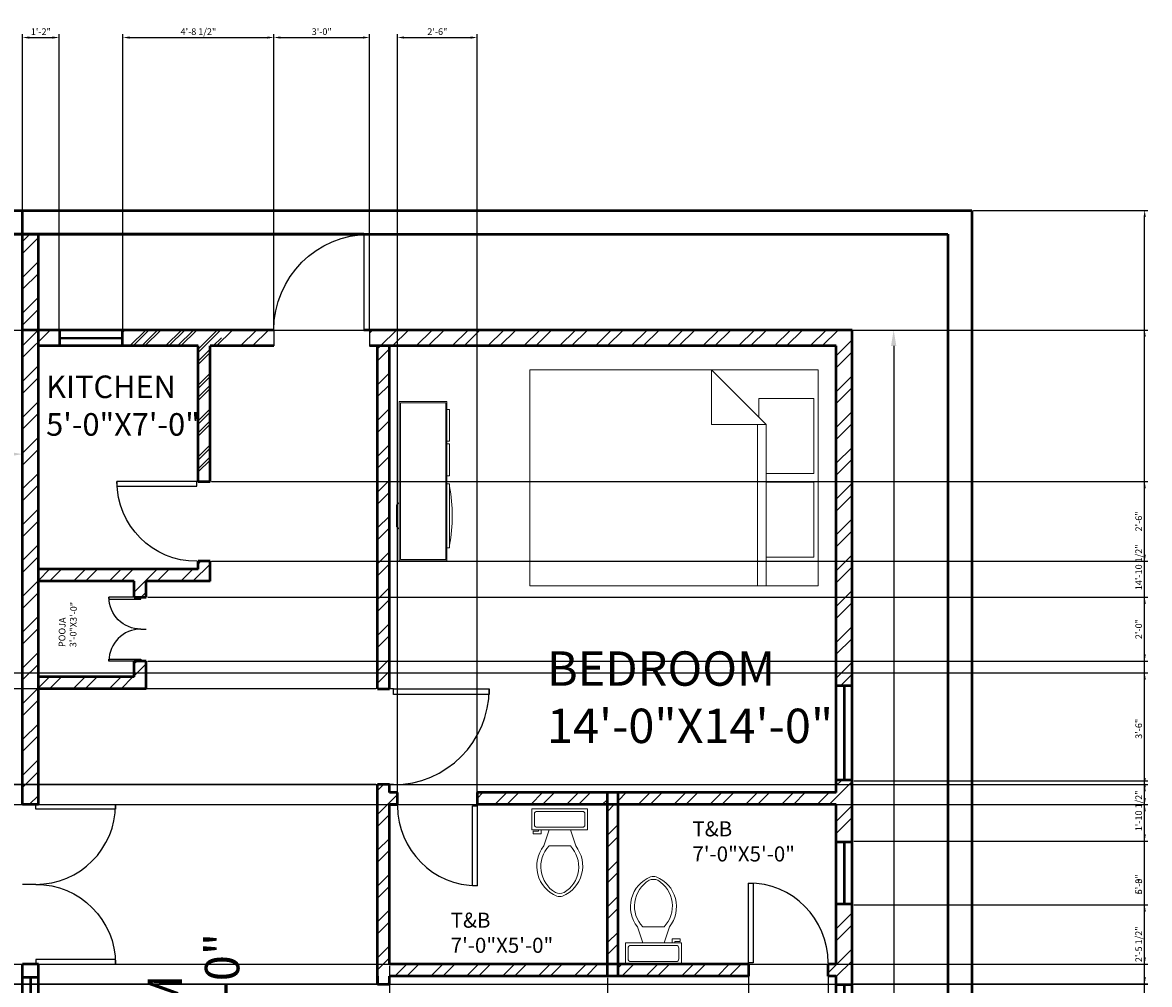
# Model space of a CAD drawing. Units: inches. Extents: x -12550 to 6516, y 1273 to 18700.
# Tile 7 of 19: x 2426 to 2849, y 2227 to 2589. Entities that reach past the tile are written whole.
import ezdxf

# ---------------------------------------------------------------- set-up
doc = ezdxf.new("R2010")
doc.units = ezdxf.units.IN
for name, color, linetype, lineweight in [('A-ANNO-DIMS', 2, 'Continuous', 18), ('A-AREA-IDEN', 1, 'Continuous', 18), ('A-DOOR', 5, 'Continuous', 25), ('A-FURN', 8, 'Continuous', 18), ('A-GLAZ', 3, 'Continuous', 25), ('A-WALL', 7, 'Continuous', 50), ('A-WALL-PATT', 8, 'Continuous', 13)]:
    doc.layers.add(name, color=color, linetype=linetype, lineweight=lineweight)
doc.styles.get("Standard").update_dxf_attribs({"font": 'arial.ttf'})
doc.dimstyles.new('ISO-25', dxfattribs={"dimtxt": 2.5, "dimasz": 2.5, "dimexe": 1.25, "dimexo": 0.625, "dimtad": 1, "dimlunit": 4, "dimtxsty": 'Standard', "dimcen": 2.5, "dimadec": 0, "dimazin": 0, "dimtfac": 1, "dimtmove": 0, "dimatfit": 3, "dimfxl": 1, "dimarcsym": 0})
pattern_1 = [(45, (-2e-13, 567), (-6.735192, 6.735192), []), (45, (4.49, 567), (-6.735192, 6.735192), [])]

# ---------------------------------------------------------------- blocks, each defined once
blk = doc.blocks.new('*U2')
for p, q in [((0, 0), (0, -5)), ((30, 0), (30, -5))]:
    blk.add_line(p, q)
blk.add_lwpolyline([(0, 0), (0, 30), (1.75, 30), (1.75, 0)], close=True)
blk.add_arc((0, 0), 30, 0, 90)
blk = doc.blocks.new('Bed - Queen')
for p, q in [((0, -80.00003), (0, 0)), ((0, 0), (59.99999, 0)), ((59.99999, 0), (59.99999, -80.00003)), ((7.99999, -1.2), (28.79998, -1.2)), ((7.99999, -14.4), (7.99999, -1.2)), ((28.79998, -1.2), (28.79998, -14.4)), ((31.19999, -1.2), (51.99999, -1.2)), ((31.19999, -14.4), (31.19999, -1.2)), ((51.99999, -1.2), (51.99999, -16.4)), ((0, -14.4), (44.8, -14.4)), ((59.99999, -29.6), (44.8, -14.4)), ((44.8, -14.4), (44.8, -29.6)), ((44.8, -16.8), (0, -16.8)), ((51.99999, -16.4), (46.79936, -16.4)), ((44.8, -29.6), (59.99999, -29.6)), ((59.99999, -80.00003), (0, -80.00003))]:
    blk.add_line(p, q)
blk = doc.blocks.new('Toilet - top')
for p, q in [((9.5, -6), (9.5, -2)), ((-8, -8.5), (-8, -8)), ((-7, -8), (-7, -9.5)), ((-4, -8), (-6, -14)), ((4, -8), (6, -14)), ((-10, -8.5), (-8, -8.5)), ((-10, -9.5), (-10, -8.5)), ((-7, -9.5), (-10, -9.5)), ((4, -14), (-4, -14))]:
    blk.add_line(p, q)
blk.add_lwpolyline([(10.5, -8), (10.5, 0), (-10.5, 0), (-10.5, -8)], close=True)
for points in [[(-9.5, -2), (-9.5, -6)], [(8.5, -1), (-8.5, -1)], [(-8.5, -7), (8.5, -7)]]:
    blk.add_lwpolyline(points)
for centre, radius, start, end in [((-8.62, -1.88), 0.884, 81.8699, 188.1301), ((8.62, -1.88), 0.884, 351.8699, 98.1301), ((-8.62, -6.12), 0.884, 171.8699, 278.1301), ((8.62, -6.12), 0.884, 261.8699, 8.1301), ((3.52, -21.58), 12.17, 141.4691, 247.9714), ((4.2, -21.82), 11.33, 136.3677, 238.9468), ((-3.52, -21.58), 12.17, 292.0284, 38.5307), ((-4.2, -21.82), 11.33, 301.053, 43.6321), ((0, -27.88), 4, 245.7318, 294.2682), ((0, -29), 4, 254.8605, 285.1395)]:
    blk.add_arc(centre, radius, start, end)
blk = doc.blocks.new('Entertainment Center')
for p, q in [((-4, 0), (-5, -1)), ((4, 0), (-4, 0)), ((5, -1), (4, 0)), ((-17, -19), (-17, -1)), ((-17, -1), (43, -1)), ((-16.5, -18.5), (-16.5, -1.5)), ((-16.5, -1.5), (42.5, -1.5)), ((42.5, -1.5), (42.5, -18.5)), ((43, -1), (43, -19)), ((43, -19), (-17, -19)), ((42.5, -18.5), (-16.5, -18.5)), ((-12, -20), (-12, -19)), ((12, -20), (-12, -20)), ((12, -19), (12, -20)), ((15, -20), (15, -19)), ((27, -20), (15, -20)), ((27, -19), (27, -20)), ((28, -20), (28, -19)), ((40, -20), (28, -20)), ((40, -19), (40, -20))]:
    blk.add_line(p, q)
blk.add_arc((0, 40), 61, 259.6111, 280.3889)
blk = doc.blocks.new('*D16')
at = {"layer": 'A-ANNO-DIMS', "color": 0, "lineweight": -2, "transparency": 16777216}
for p, q in [((2738.31, 2473.25), (2754.56, 2473.25)), ((2753.31, 2467.25), (2753.31, 1495.25)), ((2738.31, 1489.25), (2754.56, 1489.25))]:
    blk.add_line(p, q, dxfattribs=at)
at = {"layer": 'A-ANNO-DIMS', "color": 0, "transparency": 16777216}
for points in [[(2752.31, 2467.25), (2754.31, 2467.25), (2753.31, 2473.25)], [(2752.31, 1495.25), (2754.31, 1495.25), (2753.31, 1489.25)]]:
    blk.add_solid(points, dxfattribs=at)
at = {"layer": 'Defpoints', "color": 0, "transparency": 16777216}
for p in [(2737.69, 2473.25), (2737.69, 1489.25), (2753.31, 1489.25)]:
    blk.add_point(p, dxfattribs=at)
at = {"layer": 'A-ANNO-DIMS', "color": 0, "transparency": 16777216, "insert": (2749.62, 1981.25), "char_height": 6, "attachment_point": 5, "rotation": 90}
blk.add_mtext("82'", dxfattribs=at)
blk = doc.blocks.new('*D19')
at = {"layer": 'A-ANNO-DIMS', "color": 0, "lineweight": -2, "transparency": 16777216}
for p, q in [((2329.69, 2407.12), (2329.69, 2427.81)), ((2335.69, 2426.56), (2419.69, 2426.56)), ((2425.69, 2407.12), (2425.69, 2427.81))]:
    blk.add_line(p, q, dxfattribs=at)
at = {"layer": 'A-ANNO-DIMS', "color": 0, "transparency": 16777216}
for points in [[(2335.69, 2427.56), (2335.69, 2425.56), (2329.69, 2426.56)], [(2419.69, 2427.56), (2419.69, 2425.56), (2425.69, 2426.56)]]:
    blk.add_solid(points, dxfattribs=at)
at = {"layer": 'Defpoints', "color": 0, "transparency": 16777216}
for p in [(2425.69, 2426.56), (2329.69, 2406.5), (2425.69, 2406.5)]:
    blk.add_point(p, dxfattribs=at)
at = {"layer": 'A-ANNO-DIMS', "color": 0, "transparency": 16777216, "insert": (2377.69, 2430.25), "char_height": 6, "attachment_point": 5}
blk.add_mtext("8'", dxfattribs=at)
blk = doc.blocks.new('WIN-3FT')
for p, q in [((0, 0), (0, 6)), ((0, 6), (36.02, 6)), ((0.5, 0), (0.5, 6)), ((35.52, 6), (35.52, 0)), ((36.02, 6), (36.02, 0)), ((36.02, 0), (0, 0)), ((35.52, 3.2), (0.5, 3.2)), ((35.52, 2.8), (0.5, 2.8))]:
    blk.add_line(p, q)
blk = doc.blocks.new('WIN-2FT')
for p, q in [((0, 0), (0, 24.02)), ((0, 24.02), (6, 24.02)), ((0, 23.52), (6, 23.52)), ((2.8, 0.5), (2.8, 23.52)), ((3.2, 0.5), (3.2, 23.52)), ((6, 24.02), (6, 0)), ((6, 0.5), (0, 0.5)), ((6, 0), (0, 0))]:
    blk.add_line(p, q)
blk = doc.blocks.new('*D95')
at = {"layer": 'A-ANNO-DIMS', "color": 0, "lineweight": -2, "transparency": 16777216}
for p, q in [((2783.31, 2518.25), (2848.94, 2518.25)), ((2847.69, 1446.75), (2847.69, 2515.75)), ((2783.31, 1444.25), (2848.94, 1444.25))]:
    blk.add_line(p, q, dxfattribs=at)
at = {"layer": 'A-ANNO-DIMS', "color": 0, "transparency": 16777216}
for points in [[(2847.27, 2515.75), (2848.11, 2515.75), (2847.69, 2518.25)], [(2847.27, 1446.75), (2848.11, 1446.75), (2847.69, 1444.25)]]:
    blk.add_solid(points, dxfattribs=at)
at = {"layer": 'Defpoints', "color": 0, "transparency": 16777216}
for p in [(2782.69, 2518.25), (2847.69, 2518.25), (2782.69, 1444.25)]:
    blk.add_point(p, dxfattribs=at)
at = {"layer": 'A-ANNO-DIMS', "color": 0, "transparency": 16777216, "insert": (2845.79, 1981.25), "char_height": 2.5, "attachment_point": 5, "rotation": 90}
blk.add_mtext('89\'-6"', dxfattribs=at)
blk = doc.blocks.new('*D139')
at = {"layer": 'A-ANNO-DIMS', "color": 0, "lineweight": -2, "transparency": 16777216}
for p, q in [((2196.81, 2302.25), (2848.94, 2302.25)), ((2847.69, 2229.75), (2847.69, 2299.75)), ((2196.81, 2227.25), (2848.94, 2227.25))]:
    blk.add_line(p, q, dxfattribs=at)
at = {"layer": 'A-ANNO-DIMS', "color": 0, "transparency": 16777216}
for points in [[(2847.27, 2299.75), (2848.11, 2299.75), (2847.69, 2302.25)], [(2847.27, 2229.75), (2848.11, 2229.75), (2847.69, 2227.25)]]:
    blk.add_solid(points, dxfattribs=at)
at = {"layer": 'Defpoints', "color": 0, "transparency": 16777216}
for p in [(2196.19, 2302.25), (2847.69, 2302.25), (2196.19, 2227.25)]:
    blk.add_point(p, dxfattribs=at)
at = {"layer": 'A-ANNO-DIMS', "color": 0, "transparency": 16777216, "insert": (2845.79, 2264.75), "char_height": 2.5, "attachment_point": 5, "rotation": 90}
blk.add_mtext('6\'-3"', dxfattribs=at)
blk = doc.blocks.new('*D140')
at = {"layer": 'A-ANNO-DIMS', "color": 0, "lineweight": -2, "transparency": 16777216}
for p, q in [((2196.81, 2344.25), (2848.94, 2344.25)), ((2847.69, 2304.75), (2847.69, 2341.75)), ((2196.81, 2302.25), (2848.94, 2302.25))]:
    blk.add_line(p, q, dxfattribs=at)
at = {"layer": 'A-ANNO-DIMS', "color": 0, "transparency": 16777216}
for points in [[(2847.27, 2341.75), (2848.11, 2341.75), (2847.69, 2344.25)], [(2847.27, 2304.75), (2848.11, 2304.75), (2847.69, 2302.25)]]:
    blk.add_solid(points, dxfattribs=at)
at = {"layer": 'Defpoints', "color": 0, "transparency": 16777216}
for p in [(2196.19, 2344.25), (2847.69, 2344.25), (2196.19, 2302.25)]:
    blk.add_point(p, dxfattribs=at)
at = {"layer": 'A-ANNO-DIMS', "color": 0, "transparency": 16777216, "insert": (2845.79, 2323.25), "char_height": 2.5, "attachment_point": 5, "rotation": 90}
blk.add_mtext('3\'-6"', dxfattribs=at)
blk = doc.blocks.new('*D144')
at = {"layer": 'A-ANNO-DIMS', "color": 0, "lineweight": -2, "transparency": 16777216}
for p, q in [((2330.31, 2294.75), (2848.94, 2294.75)), ((2847.69, 2237.25), (2847.69, 2292.25)), ((2330.31, 2234.75), (2848.94, 2234.75))]:
    blk.add_line(p, q, dxfattribs=at)
at = {"layer": 'A-ANNO-DIMS', "color": 0, "transparency": 16777216}
for points in [[(2847.27, 2292.25), (2848.11, 2292.25), (2847.69, 2294.75)], [(2847.27, 2237.25), (2848.11, 2237.25), (2847.69, 2234.75)]]:
    blk.add_solid(points, dxfattribs=at)
at = {"layer": 'Defpoints', "color": 0, "transparency": 16777216}
for p in [(2329.69, 2294.75), (2847.69, 2294.75), (2329.69, 2234.75)]:
    blk.add_point(p, dxfattribs=at)
at = {"layer": 'A-ANNO-DIMS', "color": 0, "transparency": 16777216, "insert": (2845.79, 2264.75), "char_height": 2.5, "attachment_point": 5, "rotation": 90}
blk.add_mtext('5\'-0"', dxfattribs=at)
blk = doc.blocks.new('*D146')
at = {"layer": 'A-ANNO-DIMS', "color": 0, "lineweight": -2, "transparency": 16777216}
for p, q in [((2330.31, 2473.25), (2848.94, 2473.25)), ((2847.69, 2297.25), (2847.69, 2470.75)), ((2330.31, 2294.75), (2848.94, 2294.75))]:
    blk.add_line(p, q, dxfattribs=at)
at = {"layer": 'A-ANNO-DIMS', "color": 0, "transparency": 16777216}
for points in [[(2847.27, 2470.75), (2848.11, 2470.75), (2847.69, 2473.25)], [(2847.27, 2297.25), (2848.11, 2297.25), (2847.69, 2294.75)]]:
    blk.add_solid(points, dxfattribs=at)
at = {"layer": 'Defpoints', "color": 0, "transparency": 16777216}
for p in [(2329.69, 2473.25), (2847.69, 2473.25), (2329.69, 2294.75)]:
    blk.add_point(p, dxfattribs=at)
at = {"layer": 'A-ANNO-DIMS', "color": 0, "transparency": 16777216, "insert": (2845.77, 2384), "char_height": 2.5, "attachment_point": 5, "rotation": 90}
blk.add_mtext('14\'-10 1/2"', dxfattribs=at)
blk = doc.blocks.new('*D149')
at = {"layer": 'A-ANNO-DIMS', "color": 0, "lineweight": -2, "transparency": 16777216}
for p, q in [((2425.69, 2473.87), (2425.69, 2584.5)), ((2428.19, 2583.25), (2436.95, 2583.25)), ((2439.45, 2473.87), (2439.45, 2584.5))]:
    blk.add_line(p, q, dxfattribs=at)
at = {"layer": 'A-ANNO-DIMS', "color": 0, "transparency": 16777216}
for points in [[(2428.19, 2583.66), (2428.19, 2582.83), (2425.69, 2583.25)], [(2436.95, 2583.66), (2436.95, 2582.83), (2439.45, 2583.25)]]:
    blk.add_solid(points, dxfattribs=at)
at = {"layer": 'Defpoints', "color": 0, "transparency": 16777216}
for p in [(2439.45, 2583.25), (2425.69, 2473.25), (2439.45, 2473.25)]:
    blk.add_point(p, dxfattribs=at)
at = {"layer": 'A-ANNO-DIMS', "color": 0, "transparency": 16777216, "insert": (2432.57, 2585.13), "char_height": 2.5, "attachment_point": 5}
blk.add_mtext('1\'-2"', dxfattribs=at)
blk = doc.blocks.new('*D150')
at = {"layer": 'A-ANNO-DIMS', "color": 0, "lineweight": -2, "transparency": 16777216}
for p, q in [((2463.46, 2473.87), (2463.46, 2584.5)), ((2465.96, 2583.25), (2517.69, 2583.25)), ((2520.19, 2473.87), (2520.19, 2584.5))]:
    blk.add_line(p, q, dxfattribs=at)
at = {"layer": 'A-ANNO-DIMS', "color": 0, "transparency": 16777216}
for points in [[(2465.96, 2583.66), (2465.96, 2582.83), (2463.46, 2583.25)], [(2517.69, 2583.66), (2517.69, 2582.83), (2520.19, 2583.25)]]:
    blk.add_solid(points, dxfattribs=at)
at = {"layer": 'Defpoints', "color": 0, "transparency": 16777216}
for p in [(2520.19, 2583.25), (2463.46, 2473.25), (2520.19, 2473.25)]:
    blk.add_point(p, dxfattribs=at)
at = {"layer": 'A-ANNO-DIMS', "color": 0, "transparency": 16777216, "insert": (2491.83, 2585.16), "char_height": 2.5, "attachment_point": 5}
blk.add_mtext('4\'-8 1/2"', dxfattribs=at)
blk = doc.blocks.new('*D151')
at = {"layer": 'A-ANNO-DIMS', "color": 0, "lineweight": -2, "transparency": 16777216}
for p, q in [((2520.19, 2473.87), (2520.19, 2584.5)), ((2522.69, 2583.25), (2553.69, 2583.25)), ((2556.19, 2473.87), (2556.19, 2584.5))]:
    blk.add_line(p, q, dxfattribs=at)
at = {"layer": 'A-ANNO-DIMS', "color": 0, "transparency": 16777216}
for points in [[(2522.69, 2583.66), (2522.69, 2582.83), (2520.19, 2583.25)], [(2553.69, 2583.66), (2553.69, 2582.83), (2556.19, 2583.25)]]:
    blk.add_solid(points, dxfattribs=at)
at = {"layer": 'Defpoints', "color": 0, "transparency": 16777216}
for p in [(2556.19, 2583.25), (2520.19, 2473.25), (2556.19, 2473.25)]:
    blk.add_point(p, dxfattribs=at)
at = {"layer": 'A-ANNO-DIMS', "color": 0, "transparency": 16777216, "insert": (2538.19, 2585.15), "char_height": 2.5, "attachment_point": 5}
blk.add_mtext('3\'-0"', dxfattribs=at)
blk = doc.blocks.new('*D155')
at = {"layer": 'A-ANNO-DIMS', "color": 0, "lineweight": -2, "transparency": 16777216}
for p, q in [((2738.31, 2257.02), (2848.94, 2257.02)), ((2847.69, 2229.87), (2847.69, 2254.52)), ((2738.31, 2227.37), (2848.94, 2227.37))]:
    blk.add_line(p, q, dxfattribs=at)
at = {"layer": 'A-ANNO-DIMS', "color": 0, "transparency": 16777216}
for points in [[(2847.27, 2254.52), (2848.11, 2254.52), (2847.69, 2257.02)], [(2847.27, 2229.87), (2848.11, 2229.87), (2847.69, 2227.37)]]:
    blk.add_solid(points, dxfattribs=at)
at = {"layer": 'Defpoints', "color": 0, "transparency": 16777216}
for p in [(2737.69, 2257.02), (2847.69, 2257.02), (2737.69, 2227.37)]:
    blk.add_point(p, dxfattribs=at)
at = {"layer": 'A-ANNO-DIMS', "color": 0, "transparency": 16777216, "insert": (2845.77, 2242.2), "char_height": 2.5, "attachment_point": 5, "rotation": 90}
blk.add_mtext('2\'-5 1/2"', dxfattribs=at)
blk = doc.blocks.new('*D156')
at = {"layer": 'A-ANNO-DIMS', "color": 0, "lineweight": -2, "transparency": 16777216}
for p, q in [((2738.31, 2303.73), (2848.94, 2303.73)), ((2847.69, 2283.54), (2847.69, 2301.23)), ((2738.31, 2281.04), (2848.94, 2281.04))]:
    blk.add_line(p, q, dxfattribs=at)
at = {"layer": 'A-ANNO-DIMS', "color": 0, "transparency": 16777216}
for points in [[(2847.27, 2301.23), (2848.11, 2301.23), (2847.69, 2303.73)], [(2847.27, 2283.54), (2848.11, 2283.54), (2847.69, 2281.04)]]:
    blk.add_solid(points, dxfattribs=at)
at = {"layer": 'Defpoints', "color": 0, "transparency": 16777216}
for p in [(2737.69, 2303.73), (2847.69, 2303.73), (2737.69, 2281.04)]:
    blk.add_point(p, dxfattribs=at)
at = {"layer": 'A-ANNO-DIMS', "color": 0, "transparency": 16777216, "insert": (2845.77, 2292.39), "char_height": 2.5, "attachment_point": 5, "rotation": 90}
blk.add_mtext('1\'-10 1/2"', dxfattribs=at)
blk = doc.blocks.new('*D158')
at = {"layer": 'A-ANNO-DIMS', "color": 0, "lineweight": -2, "transparency": 16777216}
for p, q in [((2558.56, 2227.25), (1906.44, 2227.25)), ((1907.69, 2193.75), (1907.69, 2224.75)), ((2558.56, 2191.25), (1906.44, 2191.25))]:
    blk.add_line(p, q, dxfattribs=at)
at = {"layer": 'A-ANNO-DIMS', "color": 0, "transparency": 16777216}
for points in [[(1907.27, 2224.75), (1908.11, 2224.75), (1907.69, 2227.25)], [(1907.27, 2193.75), (1908.11, 2193.75), (1907.69, 2191.25)]]:
    blk.add_solid(points, dxfattribs=at)
at = {"layer": 'Defpoints', "color": 0, "transparency": 16777216}
for p in [(1907.69, 2227.25), (2559.19, 2227.25), (2559.19, 2191.25)]:
    blk.add_point(p, dxfattribs=at)
at = {"layer": 'A-ANNO-DIMS', "color": 0, "transparency": 16777216, "insert": (1905.79, 2209.25), "char_height": 2.5, "attachment_point": 5, "rotation": 90}
blk.add_mtext('3\'-0"', dxfattribs=at)
blk = doc.blocks.new('*D159')
at = {"layer": 'A-ANNO-DIMS', "color": 0, "lineweight": -2, "transparency": 16777216}
for p, q in [((2558.56, 2302.25), (1906.44, 2302.25)), ((1907.69, 2229.75), (1907.69, 2299.75)), ((2558.56, 2227.25), (1906.44, 2227.25))]:
    blk.add_line(p, q, dxfattribs=at)
at = {"layer": 'A-ANNO-DIMS', "color": 0, "transparency": 16777216}
for points in [[(1907.27, 2299.75), (1908.11, 2299.75), (1907.69, 2302.25)], [(1907.27, 2229.75), (1908.11, 2229.75), (1907.69, 2227.25)]]:
    blk.add_solid(points, dxfattribs=at)
at = {"layer": 'Defpoints', "color": 0, "transparency": 16777216}
for p in [(1907.69, 2302.25), (2559.19, 2302.25), (2559.19, 2227.25)]:
    blk.add_point(p, dxfattribs=at)
at = {"layer": 'A-ANNO-DIMS', "color": 0, "transparency": 16777216, "insert": (1905.79, 2264.75), "char_height": 2.5, "attachment_point": 5, "rotation": 90}
blk.add_mtext('6\'-3"', dxfattribs=at)
blk = doc.blocks.new('*D160')
at = {"layer": 'A-ANNO-DIMS', "color": 0, "lineweight": -2, "transparency": 16777216}
for p, q in [((2558.56, 2338.25), (1906.44, 2338.25)), ((1907.69, 2304.75), (1907.69, 2335.75)), ((2558.56, 2302.25), (1906.44, 2302.25))]:
    blk.add_line(p, q, dxfattribs=at)
at = {"layer": 'A-ANNO-DIMS', "color": 0, "transparency": 16777216}
for points in [[(1907.27, 2335.75), (1908.11, 2335.75), (1907.69, 2338.25)], [(1907.27, 2304.75), (1908.11, 2304.75), (1907.69, 2302.25)]]:
    blk.add_solid(points, dxfattribs=at)
at = {"layer": 'Defpoints', "color": 0, "transparency": 16777216}
for p in [(1907.69, 2338.25), (2559.19, 2338.25), (2559.19, 2302.25)]:
    blk.add_point(p, dxfattribs=at)
at = {"layer": 'A-ANNO-DIMS', "color": 0, "transparency": 16777216, "insert": (1905.79, 2320.25), "char_height": 2.5, "attachment_point": 5, "rotation": 90}
blk.add_mtext('3\'-0"', dxfattribs=at)
blk = doc.blocks.new('*D161')
at = {"layer": 'A-ANNO-DIMS', "color": 0, "lineweight": -2, "transparency": 16777216}
for p, q in [((2566.69, 2295.37), (2566.69, 2584.5)), ((2569.19, 2583.25), (2594.19, 2583.25)), ((2596.69, 2295.37), (2596.69, 2584.5))]:
    blk.add_line(p, q, dxfattribs=at)
at = {"layer": 'A-ANNO-DIMS', "color": 0, "transparency": 16777216}
for points in [[(2569.19, 2583.66), (2569.19, 2582.83), (2566.69, 2583.25)], [(2594.19, 2583.66), (2594.19, 2582.83), (2596.69, 2583.25)]]:
    blk.add_solid(points, dxfattribs=at)
at = {"layer": 'Defpoints', "color": 0, "transparency": 16777216}
for p in [(2596.69, 2583.25), (2566.69, 2294.75), (2596.69, 2294.75)]:
    blk.add_point(p, dxfattribs=at)
at = {"layer": 'A-ANNO-DIMS', "color": 0, "transparency": 16777216, "insert": (2581.69, 2585.15), "char_height": 2.5, "attachment_point": 5}
blk.add_mtext('2\'-6"', dxfattribs=at)
blk = doc.blocks.new('*D162')
at = {"layer": 'A-ANNO-DIMS', "color": 0, "lineweight": -2, "transparency": 16777216}
for p, q in [((2698.69, 2234.12), (2698.69, 1378)), ((2728.69, 2234.12), (2728.69, 1378)), ((2701.19, 1379.25), (2726.19, 1379.25))]:
    blk.add_line(p, q, dxfattribs=at)
at = {"layer": 'A-ANNO-DIMS', "color": 0, "transparency": 16777216}
for points in [[(2701.19, 1379.66), (2701.19, 1378.83), (2698.69, 1379.25)], [(2726.19, 1379.66), (2726.19, 1378.83), (2728.69, 1379.25)]]:
    blk.add_solid(points, dxfattribs=at)
at = {"layer": 'Defpoints', "color": 0, "transparency": 16777216}
for p in [(2698.69, 2234.75), (2728.69, 2234.75), (2728.69, 1379.25)]:
    blk.add_point(p, dxfattribs=at)
at = {"layer": 'A-ANNO-DIMS', "color": 0, "transparency": 16777216, "insert": (2713.69, 1381.15), "char_height": 2.5, "attachment_point": 5}
blk.add_mtext('2\'-6"', dxfattribs=at)
blk = doc.blocks.new('*D163')
at = {"layer": 'A-ANNO-DIMS', "color": 0, "lineweight": -2, "transparency": 16777216}
for p, q in [((2563.69, 2234.12), (2563.69, 1378)), ((2645.69, 2229.62), (2645.69, 1378)), ((2566.19, 1379.25), (2643.19, 1379.25))]:
    blk.add_line(p, q, dxfattribs=at)
at = {"layer": 'A-ANNO-DIMS', "color": 0, "transparency": 16777216}
for points in [[(2566.19, 1379.66), (2566.19, 1378.83), (2563.69, 1379.25)], [(2643.19, 1379.66), (2643.19, 1378.83), (2645.69, 1379.25)]]:
    blk.add_solid(points, dxfattribs=at)
at = {"layer": 'Defpoints', "color": 0, "transparency": 16777216}
for p in [(2563.69, 2234.75), (2645.69, 2230.25), (2645.69, 1379.25)]:
    blk.add_point(p, dxfattribs=at)
at = {"layer": 'A-ANNO-DIMS', "color": 0, "transparency": 16777216, "insert": (2604.69, 1381.15), "char_height": 2.5, "attachment_point": 5}
blk.add_mtext('6\'-10"', dxfattribs=at)
blk = doc.blocks.new('*D167')
at = {"layer": 'A-ANNO-DIMS', "color": 0, "lineweight": -2, "transparency": 16777216}
for p, q in [((2496.81, 2416.25), (2848.94, 2416.25)), ((2847.69, 2388.75), (2847.69, 2413.75)), ((2496.81, 2386.25), (2848.94, 2386.25))]:
    blk.add_line(p, q, dxfattribs=at)
at = {"layer": 'A-ANNO-DIMS', "color": 0, "transparency": 16777216}
for points in [[(2847.27, 2413.75), (2848.11, 2413.75), (2847.69, 2416.25)], [(2847.27, 2388.75), (2848.11, 2388.75), (2847.69, 2386.25)]]:
    blk.add_solid(points, dxfattribs=at)
at = {"layer": 'Defpoints', "color": 0, "transparency": 16777216}
for p in [(2496.19, 2416.25), (2847.69, 2416.25), (2496.19, 2386.25)]:
    blk.add_point(p, dxfattribs=at)
at = {"layer": 'A-ANNO-DIMS', "color": 0, "transparency": 16777216, "insert": (2845.79, 2401.25), "char_height": 2.5, "attachment_point": 5, "rotation": 90}
blk.add_mtext('2\'-6"', dxfattribs=at)
blk = doc.blocks.new('*D168')
at = {"layer": 'A-ANNO-DIMS', "color": 0, "lineweight": -2, "transparency": 16777216}
for p, q in [((2472.81, 2372.75), (2848.94, 2372.75)), ((2847.69, 2351.25), (2847.69, 2370.25)), ((2472.81, 2348.75), (2848.94, 2348.75))]:
    blk.add_line(p, q, dxfattribs=at)
at = {"layer": 'A-ANNO-DIMS', "color": 0, "transparency": 16777216}
for points in [[(2847.27, 2370.25), (2848.11, 2370.25), (2847.69, 2372.75)], [(2847.27, 2351.25), (2848.11, 2351.25), (2847.69, 2348.75)]]:
    blk.add_solid(points, dxfattribs=at)
at = {"layer": 'Defpoints', "color": 0, "transparency": 16777216}
for p in [(2472.19, 2372.75), (2847.69, 2372.75), (2472.19, 2348.75)]:
    blk.add_point(p, dxfattribs=at)
at = {"layer": 'A-ANNO-DIMS', "color": 0, "transparency": 16777216, "insert": (2845.79, 2360.75), "char_height": 2.5, "attachment_point": 5, "rotation": 90}
blk.add_mtext('2\'-0"', dxfattribs=at)

msp = doc.modelspace()

# ---------------------------------------------------------------- hatches: boundary and pattern name
at = {"layer": 'A-WALL-PATT'}
h = msp.add_hatch(dxfattribs=at)
h.set_pattern_fill('ANSI32', color=256)
h.paths.add_polyline_path([(2431.689, 2509.247), (2425.689, 2509.247), (2425.689, 2473.247), (2431.689, 2473.247)])
h = msp.add_hatch(dxfattribs=at)
h.set_pattern_fill('ANSI32', color=256)
h.set_pattern_definition(pattern_1)
h.paths.add_polyline_path([(2439.446, 2473.247), (2425.689, 2473.247), (2425.689, 2294.747), (2430.689, 2294.747), (2431.689, 2294.747), (2431.689, 2467.247), (2439.446, 2467.247)])
h = msp.add_hatch(dxfattribs=at)
h.set_pattern_fill('ANSI32', color=256)
h.set_pattern_definition(pattern_1)
h.paths.add_polyline_path([(2500.528, 2473.247), (2463.463, 2473.247), (2463.463, 2467.247), (2491.689, 2467.247), (2491.689, 2416.247), (2496.189, 2416.247), (2496.189, 2467.247), (2500.528, 2467.247)])
h = msp.add_hatch(dxfattribs=at)
h.set_pattern_fill('ANSI32', color=256)
h.paths.add_polyline_path([(2463.463, 2473.247), (2463.463, 2467.247), (2491.689, 2467.247), (2491.689, 2416.247), (2496.189, 2416.247), (2496.189, 2467.247), (2520.189, 2467.247), (2520.189, 2473.247)])
h = msp.add_hatch(dxfattribs=at)
h.set_pattern_fill('ANSI32', color=256)
h.set_pattern_definition(pattern_1)
h.paths.add_polyline_path([(2556.189, 2473.247), (2556.189, 2467.247), (2731.689, 2467.247), (2731.689, 2339.747), (2737.689, 2339.747), (2737.689, 2473.247)])
h = msp.add_hatch(dxfattribs=at)
h.set_pattern_fill('ANSI32', color=256)
h.set_pattern_definition(pattern_1)
h.paths.add_polyline_path([(2563.689, 2467.247), (2559.189, 2467.247), (2559.189, 2338.247), (2563.689, 2338.247)])
h = msp.add_hatch(dxfattribs=at)
h.set_pattern_fill('ANSI32', color=256)
h.set_pattern_definition(pattern_1)
h.paths.add_polyline_path([(2496.189, 2386.247), (2491.689, 2386.247), (2491.689, 2383.247), (2431.689, 2383.247), (2431.689, 2378.747), (2467.689, 2378.747), (2467.689, 2372.747), (2470.189, 2372.747), (2472.189, 2372.747), (2472.189, 2378.747), (2496.189, 2378.747)])
h = msp.add_hatch(dxfattribs=at)
h.set_pattern_fill('ANSI32', color=256)
h.set_pattern_definition(pattern_1)
h.paths.add_polyline_path([(2472.189, 2348.747), (2470.189, 2348.747), (2467.689, 2348.747), (2467.689, 2342.747), (2431.689, 2342.747), (2431.689, 2338.247), (2472.189, 2338.247)])
h = msp.add_hatch(dxfattribs=at)
h.set_pattern_fill('ANSI32', color=256)
h.set_pattern_definition(pattern_1)
h.paths.add_polyline_path([(2563.689, 2294.747), (2566.689, 2294.747), (2566.689, 2299.247), (2563.689, 2299.247), (2563.689, 2302.247), (2559.189, 2302.247), (2559.189, 2227.247), (2563.689, 2227.247), (2563.689, 2230.247), (2566.641, 2230.247), (2645.689, 2230.247), (2645.689, 2234.747), (2566.641, 2234.747), (2563.689, 2234.747)])
h = msp.add_hatch(dxfattribs=at)
h.set_pattern_fill('ANSI32', color=256)
h.set_pattern_definition(pattern_1)
h.paths.add_polyline_path([(2737.689, 2303.73), (2731.689, 2303.73), (2731.689, 2299.247), (2728.689, 2299.247), (2649.689, 2299.247), (2649.689, 2294.747), (2728.689, 2294.747), (2731.689, 2294.747), (2731.689, 2281.042), (2737.689, 2281.042)])
h = msp.add_hatch(dxfattribs=at)
h.set_pattern_fill('ANSI32', color=256)
h.set_pattern_definition(pattern_1)
h.paths.add_polyline_path([(2645.689, 2299.247), (2596.689, 2299.247), (2596.689, 2294.747), (2645.689, 2294.747)], flags=17)
h = msp.add_hatch(dxfattribs=at)
h.set_pattern_fill('ANSI32', color=256)
h.set_pattern_definition(pattern_1)
h.paths.add_polyline_path([(2649.689, 2294.747), (2645.689, 2294.747), (2645.689, 2234.747), (2649.689, 2234.747)])
h = msp.add_hatch(dxfattribs=at)
h.set_pattern_fill('ANSI32', color=256)
h.set_pattern_definition(pattern_1)
h.paths.add_polyline_path([(2737.689, 2257.024), (2731.689, 2257.024), (2731.689, 2234.747), (2728.689, 2234.747), (2728.689, 2230.247), (2731.689, 2230.247), (2731.689, 2227.369), (2737.689, 2227.369)])
h = msp.add_hatch(dxfattribs=at)
h.set_pattern_fill('ANSI32', color=256)
h.set_pattern_definition(pattern_1)
h.paths.add_polyline_path([(2698.689, 2234.747), (2649.689, 2234.747), (2649.689, 2230.247), (2698.689, 2230.247)])

# ---------------------------------------------------------------- linework, layer by layer
at = {"layer": 'A-WALL'}
for p, q in [((1972.689, 2518.247), (2782.689, 2518.247)), ((2425.689, 2294.747), (2425.689, 2518.247)), ((2782.689, 2518.247), (2782.689, 1444.247)), ((1981.689, 2509.247), (2773.689, 2509.247)), ((2554.089, 2509.247), (2254.089, 2509.247)), ((2431.689, 2294.747), (2431.689, 2509.247)), ((2773.689, 2509.247), (2773.689, 1453.247)), ((2520.189, 2473.247), (2425.689, 2473.247)), ((2559.189, 2473.247), (2554.089, 2473.247)), ((2737.689, 2473.247), (2559.189, 2473.247)), ((2737.689, 2060.923), (2737.689, 2473.247)), ((2491.689, 2467.247), (2431.689, 2467.247)), ((2491.689, 2416.247), (2491.689, 2467.247)), ((2496.189, 2416.247), (2496.189, 2467.247)), ((2520.189, 2467.247), (2496.189, 2467.247)), ((2559.189, 2467.247), (2556.189, 2467.247)), ((2731.689, 2467.247), (2559.189, 2467.247)), ((2559.189, 2338.247), (2559.189, 2467.247)), ((2563.689, 2338.247), (2563.689, 2467.247)), ((2731.689, 2299.247), (2731.689, 2467.247)), ((2491.689, 2416.247), (2496.189, 2416.247)), ((2491.689, 2383.247), (2491.689, 2386.247)), ((2496.189, 2386.247), (2491.689, 2386.247)), ((2496.189, 2378.747), (2496.189, 2386.247)), ((2496.189, 2383.247), (2496.189, 2386.247)), ((2491.689, 2383.247), (2431.689, 2383.247)), ((2467.689, 2378.747), (2431.689, 2378.747)), ((2467.689, 2372.747), (2467.689, 2378.747)), ((2496.189, 2378.747), (2472.189, 2378.747)), ((2472.189, 2372.747), (2472.189, 2378.747)), ((2467.689, 2372.747), (2472.189, 2372.747)), ((2467.689, 2342.747), (2467.689, 2348.747)), ((2472.189, 2348.747), (2467.689, 2348.747)), ((2472.189, 2338.247), (2472.189, 2348.747)), ((2472.189, 2342.747), (2472.189, 2348.747)), ((2467.689, 2342.747), (2431.689, 2342.747)), ((2472.189, 2338.247), (2431.689, 2338.247)), ((2559.189, 2338.247), (2563.689, 2338.247)), ((2559.189, 2227.247), (2559.189, 2302.247)), ((2563.689, 2302.247), (2559.189, 2302.247)), ((2563.689, 2299.247), (2563.689, 2302.247)), ((2563.689, 2299.247), (2563.689, 2302.247)), ((2563.689, 2299.247), (2563.689, 2302.247)), ((2563.689, 2299.247), (2563.689, 2302.247)), ((2566.689, 2299.247), (2563.689, 2299.247)), ((2566.689, 2294.747), (2566.689, 2299.247)), ((2728.689, 2299.247), (2596.689, 2299.247)), ((2596.689, 2299.247), (2596.689, 2294.747)), ((2645.689, 2230.247), (2645.689, 2299.247)), ((2649.689, 2230.247), (2649.689, 2299.247)), ((2731.689, 2299.247), (2728.689, 2299.247)), ((2731.689, 2299.247), (2728.689, 2299.247)), ((2431.689, 2294.747), (2425.689, 2294.747)), ((2566.689, 2294.747), (2563.689, 2294.747)), ((2563.689, 2234.747), (2563.689, 2294.747)), ((2563.689, 2234.747), (2563.689, 2294.747)), ((2563.689, 2234.747), (2563.689, 2294.747)), ((2563.689, 2294.747), (2566.689, 2294.747)), ((2728.689, 2294.747), (2596.689, 2294.747)), ((2731.689, 2294.747), (2728.689, 2294.747)), ((2731.689, 2234.747), (2731.689, 2294.747)), ((2431.689, 2234.747), (2425.689, 2234.747)), ((2425.689, 2056.247), (2425.689, 2234.747)), ((2431.689, 2062.247), (2431.689, 2234.747)), ((2566.641, 2234.747), (2563.689, 2234.747)), ((2698.689, 2234.747), (2566.641, 2234.747)), ((2698.689, 2234.747), (2698.689, 2230.247)), ((2731.689, 2234.747), (2728.689, 2234.747)), ((2728.689, 2230.247), (2728.689, 2234.747)), ((2559.189, 2230.247), (2559.189, 2227.247)), ((2566.641, 2230.247), (2563.689, 2230.247)), ((2563.689, 2227.247), (2563.689, 2230.247)), ((2563.689, 2227.247), (2563.689, 2230.247)), ((2563.689, 2227.247), (2563.689, 2230.247)), ((2698.689, 2230.247), (2566.641, 2230.247)), ((2731.689, 2230.247), (2728.689, 2230.247)), ((2731.689, 2230.247), (2728.689, 2230.247)), ((2731.689, 2062.247), (2731.689, 2230.247)), ((2559.189, 2227.247), (2563.689, 2227.247))]:
    msp.add_line(p, q, dxfattribs=at)

# ---------------------------------------------------------------- block references
at = {"layer": 'A-DOOR', "xscale": -1.199999999999999, "yscale": 1.199999999999999, "zscale": 1.199999999999999}
msp.add_blockref('*U2', (2556.189, 2473.247), dxfattribs=at)
at = {"layer": 'A-DOOR', "xscale": -1}
for p, rotation in [((2491.189, 2416.247), 90), ((2430.689, 2234.747), 270)]:
    msp.add_blockref('*U2', p, dxfattribs=dict(at, rotation=rotation))
at = {"layer": 'A-DOOR'}
for p, xscale, yscale, zscale, rotation in [((2470.189, 2372.747), -0.399999999999997, 0.399999999999997, 0.399999999999997, 90), ((2470.189, 2348.747), 0.399999999999997, 0.399999999999997, 0.399999999999997, 90.00000000000003), ((2565.189, 2338.247), 1.199999999999999, 1.199999999999999, 1.199999999999999, 270)]:
    msp.add_blockref('*U2', p, dxfattribs=dict(at, xscale=xscale, yscale=yscale, zscale=zscale, rotation=rotation))
for p, rotation in [((2596.689, 2294.247), 180), ((2430.689, 2294.747), 270)]:
    msp.add_blockref('*U2', p, dxfattribs=dict(at, rotation=rotation))
msp.add_blockref('*U2', (2698.689, 2235.247), dxfattribs=at)
at = {"layer": 'A-FURN', "xscale": -1.354827908062564, "yscale": 1.354827908062564, "zscale": 1.354827908062564, "rotation": 270}
msp.add_blockref('Bed - Queen', (2724.868, 2376.994), dxfattribs=at)
at = {"layer": 'A-FURN'}
for name, p, rotation in [('Entertainment Center', (2566.318, 2403.379), 89.99999999999999), ('Toilet - top', (2662.958, 2234.747), 180)]:
    msp.add_blockref(name, p, dxfattribs=dict(at, rotation=rotation))
msp.add_blockref('Toilet - top', (2627.711, 2293.198), dxfattribs=at)
at = {"layer": 'A-GLAZ'}
for name, p, rotation in [('WIN-2FT', (2439.446, 2473.247), 269.9999999999959), ('WIN-3FT', (2737.689, 2303.73), 90.00000000000072), ('WIN-2FT', (2737.689, 2281.042), 180), ('WIN-3FT', (2431.689, 2194.032), 90.00000000000047), ('WIN-3FT', (2737.689, 2191.352), 90.00000000000047)]:
    msp.add_blockref(name, p, dxfattribs=dict(at, rotation=rotation))

# ---------------------------------------------------------------- texts
at = {"layer": 'A-AREA-IDEN', "attachment_point": 1}
for s, width, gutter_width, insert, char_height in [('KITCHEN\\P5\'-0"X7\'-0"', 1.29487, 42.422, (2434.569, 2456.124), 8.48435), ('T&B\\P7\'-0"X5\'-0"', 4.19569, 28.328, (2677.611, 2288.465), 5.66556), ('T&B\\P7\'-0"X5\'-0"', 4.19569, 28.328, (2586.701, 2254.107), 5.66556)]:
    msp.add_mtext_dynamic_manual_height_columns(s, width=width, gutter_width=gutter_width, heights=[0], dxfattribs=dict(at, insert=insert, char_height=char_height))
at = {"layer": 'A-AREA-IDEN', "insert": (2439.241, 2354.026), "char_height": 2.5, "attachment_point": 1, "rotation": 89.18385}
msp.add_mtext_dynamic_manual_height_columns('POOJA\\P3\'-0"X3\'-0"', width=0.78585, gutter_width=12.5, heights=[0], dxfattribs=at)
at = {"layer": 'A-AREA-IDEN', "insert": (2622.904, 2352.378), "char_height": 12.93169, "attachment_point": 1}
msp.add_mtext('BEDROOM\\P14\'-0"X14\'-0"', dxfattribs=at)
at = {"layer": 'A-AREA-IDEN', "insert": (2472.713, 2124.153), "char_height": 12.93169, "attachment_point": 1, "rotation": 90}
msp.add_mtext('LIVINGROOM\\P10\'-7.5"X23\'-0"', dxfattribs=at)

# ---------------------------------------------------------------- dimensions: what is measured, and where the dimension line sits
at = {"layer": 'A-ANNO-DIMS'}
for base, p1, p2, override, picture, middle in [((2439.446, 2583.247), (2425.689, 2473.247), (2439.446, 2473.247), {"dimdec": 1, "dimlfac": 1, "dimrnd": 0, "dimzin": 1, "dimdsep": 46, "dimlunit": 4, "dimfrac": 2}, '*D149', (2432.567, 2585.127)), ((2520.189, 2583.247), (2463.463, 2473.247), (2520.189, 2473.247), {"dimdec": 1, "dimlfac": 1, "dimrnd": 0, "dimzin": 1, "dimdsep": 46, "dimlunit": 4, "dimfrac": 2}, '*D150', (2491.826, 2585.165)), ((2556.189, 2583.247), (2520.189, 2473.247), (2556.189, 2473.247), {"dimdec": 1, "dimlfac": 1, "dimrnd": 0, "dimzin": 1, "dimdsep": 46, "dimlunit": 4, "dimfrac": 2}, '*D151', (2538.189, 2585.15)), ((2596.689, 2583.247), (2566.689, 2294.747), (2596.689, 2294.747), {"dimdec": 1, "dimlfac": 1, "dimrnd": 0, "dimzin": 1, "dimdsep": 46, "dimlunit": 4, "dimfrac": 2}, '*D161', (2581.689, 2585.149)), ((2425.689, 2426.562), (2329.689, 2406.497), (2425.689, 2406.497), {"dimtxt": 6, "dimasz": 6, "dimclrd": 0, "dimclre": 0, "dimclrt": 0}, '*D19', (2377.689, 2430.25)), ((2645.689, 1379.247), (2563.689, 2234.747), (2645.689, 2230.247), {"dimdec": 1, "dimlfac": 1, "dimrnd": 0, "dimzin": 1, "dimdsep": 46, "dimlunit": 4, "dimfrac": 2}, '*D163', (2604.689, 1381.149)), ((2728.689, 1379.247), (2698.689, 2234.747), (2728.689, 2234.747), {"dimdec": 1, "dimlfac": 1, "dimrnd": 0, "dimzin": 1, "dimdsep": 46, "dimlunit": 4, "dimfrac": 2}, '*D162', (2713.689, 1381.149))]:
    dim = msp.add_linear_dim(base=base, p1=p1, p2=p2, dimstyle='ISO-25', override=override, dxfattribs=at)
    dim.commit()
    dim.dimension.update_dxf_attribs({"geometry": picture, "text_midpoint": middle})
for base, p1, p2, override, picture, middle in [((2847.689, 2518.247), (2782.689, 1444.247), (2782.689, 2518.247), {"dimdec": 1, "dimlfac": 1, "dimrnd": 0, "dimzin": 1, "dimdsep": 46, "dimlunit": 4, "dimfrac": 2}, '*D95', (2845.787, 1981.247)), ((2847.689, 2473.247), (2329.689, 2294.747), (2329.689, 2473.247), {"dimdec": 1, "dimlfac": 1, "dimrnd": 0, "dimzin": 1, "dimdsep": 46, "dimlunit": 4, "dimfrac": 2}, '*D146', (2845.771, 2383.997)), ((2753.309, 1489.247), (2737.689, 2473.247), (2737.689, 1489.247), {"dimtxt": 6, "dimasz": 6, "dimclrd": 0, "dimclre": 0, "dimclrt": 0}, '*D16', (2749.62, 1981.247)), ((2847.689, 2416.247), (2496.189, 2386.247), (2496.189, 2416.247), {"dimdec": 1, "dimlfac": 1, "dimrnd": 0, "dimzin": 1, "dimdsep": 46, "dimlunit": 4, "dimfrac": 2}, '*D167', (2845.787, 2401.247)), ((2847.689, 2372.747), (2472.189, 2348.747), (2472.189, 2372.747), {"dimdec": 1, "dimlfac": 1, "dimrnd": 0, "dimzin": 1, "dimdsep": 46, "dimlunit": 4, "dimfrac": 2}, '*D168', (2845.787, 2360.747)), ((2847.689, 2344.247), (2196.189, 2302.247), (2196.189, 2344.247), {"dimdec": 1, "dimlfac": 1, "dimrnd": 0, "dimzin": 1, "dimdsep": 46, "dimlunit": 4, "dimfrac": 2}, '*D140', (2845.787, 2323.247)), ((1907.689, 2338.247), (2559.189, 2302.247), (2559.189, 2338.247), {"dimdec": 1, "dimlfac": 1, "dimrnd": 0, "dimzin": 1, "dimdsep": 46, "dimlunit": 4, "dimfrac": 2}, '*D160', (1905.787, 2320.247)), ((1907.689, 2302.247), (2559.189, 2227.247), (2559.189, 2302.247), {"dimdec": 1, "dimlfac": 1, "dimrnd": 0, "dimzin": 1, "dimdsep": 46, "dimlunit": 4, "dimfrac": 2}, '*D159', (1905.787, 2264.747)), ((2847.689, 2302.247), (2196.189, 2227.247), (2196.189, 2302.247), {"dimdec": 1, "dimlfac": 1, "dimrnd": 0, "dimzin": 1, "dimdsep": 46, "dimlunit": 4, "dimfrac": 2}, '*D139', (2845.787, 2264.747)), ((2847.689, 2303.73), (2737.689, 2281.042), (2737.689, 2303.73), {"dimdec": 1, "dimlfac": 1, "dimrnd": 0, "dimzin": 1, "dimdsep": 46, "dimlunit": 4, "dimfrac": 2}, '*D156', (2845.771, 2292.386)), ((2847.689, 2294.747), (2329.689, 2234.747), (2329.689, 2294.747), {"dimdec": 1, "dimlfac": 1, "dimrnd": 0, "dimzin": 1, "dimdsep": 46, "dimlunit": 4, "dimfrac": 2}, '*D144', (2845.787, 2264.747)), ((2847.689, 2257.024), (2737.689, 2227.369), (2737.689, 2257.024), {"dimdec": 1, "dimlfac": 1, "dimrnd": 0, "dimzin": 1, "dimdsep": 46, "dimlunit": 4, "dimfrac": 2}, '*D155', (2845.771, 2242.197)), ((1907.689, 2227.247), (2559.189, 2191.247), (2559.189, 2227.247), {"dimdec": 1, "dimlfac": 1, "dimrnd": 0, "dimzin": 1, "dimdsep": 46, "dimlunit": 4, "dimfrac": 2}, '*D158', (1905.787, 2209.247))]:
    dim = msp.add_linear_dim(base=base, p1=p1, p2=p2, angle=90, dimstyle='ISO-25', override=override, dxfattribs=at)
    dim.commit()
    dim.dimension.update_dxf_attribs({"geometry": picture, "text_midpoint": middle})

doc.saveas('drawing.dxf')
